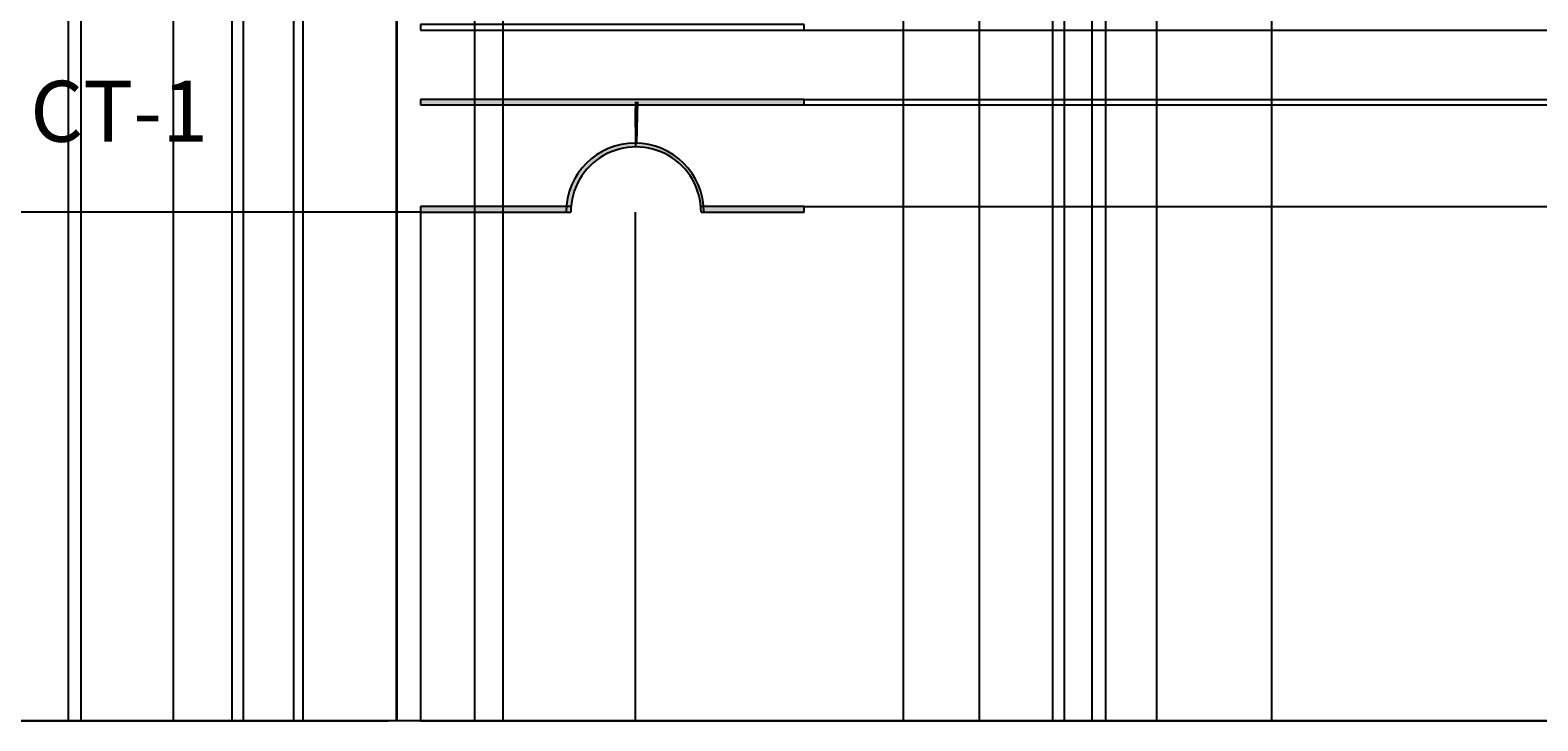
# Model space of a CAD drawing. Units: inches. Extents: x 35362 to 73946, y 43607 to 67532.
# Tile 126 of 134: x 52380 to 57838, y 43607 to 46109. Entities that reach past the tile are written whole.
import ezdxf

# ---------------------------------------------------------------- set-up
doc = ezdxf.new("R2010")
doc.units = ezdxf.units.IN
doc.header["$MEASUREMENT"] = 0
for name, color, linetype, lineweight in [('A-ANNO-DIMS', 2, 'Continuous', 18), ('E-ANNO-TEXT', 5, 'Continuous', 18), ('E-SYMB', 1, 'Continuous', 25), ('E-SYMB-PATT', 1, 'Continuous', 13)]:
    doc.layers.add(name, color=color, linetype=linetype, lineweight=lineweight)
doc.styles.get("Standard").update_dxf_attribs({"font": 'arial.ttf'})
doc.dimstyles.get("Standard").update_dxf_attribs({"dimtxt": 0.18, "dimasz": 0.18, "dimexe": 0.18, "dimexo": 0.0625, "dimgap": 0.09, "dimtad": 0, "dimtih": 1, "dimtoh": 1, "dimdec": 4, "dimzin": 0, "dimdsep": 46, "dimtxsty": 'Standard', "dimcen": 0.09, "dimadec": 0, "dimazin": 0, "dimtfac": 1, "dimtdec": 4, "dimtofl": 0, "dimtmove": 0, "dimatfit": 3, "dimfxl": 1, "dimtolj": 1, "dimtzin": 0, "dimarcsym": 0})

# ---------------------------------------------------------------- blocks, each defined once
blk = doc.blocks.new('CT-CORE')
for p, q in [((0, 1388), (0, 0)), ((20, 1388), (0, 1388)), ((20, 0), (20, 1388)), ((270.7, 1388), (270.7, 0)), ((290.7, 1388), (270.7, 1388)), ((290.7, 0), (290.7, 1388)), ((659, 1388), (659, 1014.6)), ((679, 1388), (659, 1388)), ((679, 1015.4), (679, 1388)), ((659, 544.4), (659, 0)), ((679, 0), (679, 543.5)), ((0, 0), (20, 0)), ((270.7, 0), (290.7, 0)), ((659, 0), (679, 0))]:
    blk.add_line(p, q)
blk.add_arc((679, 779.5), 235.9, 90, 270)
blk = doc.blocks.new('*D5')
at = {"layer": 'A-ANNO-DIMS', "color": 0, "lineweight": -2, "transparency": 16777216}
for p, q in [((37121.9, 46919.3), (37121.9, 43606.7)), ((69871.5, 45449.8), (69871.5, 43606.7)), ((37122.1, 43606.9), (53496.3, 43606.9)), ((69871.3, 43606.9), (53497.2, 43606.9))]:
    blk.add_line(p, q, dxfattribs=at)
at = {"layer": 'A-ANNO-DIMS', "color": 0, "transparency": 16777216}
for points in [[(37122.1, 43606.9), (37122.1, 43606.8), (37121.9, 43606.9)], [(69871.3, 43606.9), (69871.3, 43606.8), (69871.5, 43606.9)]]:
    blk.add_solid(points, dxfattribs=at)
at = {"layer": 'Defpoints', "color": 0, "transparency": 16777216}
for p in [(37121.9, 46919.4), (69871.5, 45449.9), (69871.5, 43606.9)]:
    blk.add_point(p, dxfattribs=at)
at = {"layer": 'A-ANNO-DIMS', "color": 0, "transparency": 16777216, "insert": (53496.7, 43606.9), "char_height": 0.18, "attachment_point": 5}
blk.add_mtext('\\A1;32750', dxfattribs=at)
blk = doc.blocks.new('*D11')
at = {"layer": 'A-ANNO-DIMS', "color": 0, "lineweight": -2, "transparency": 16777216}
for p, q in [((47978.7, 56028.8), (47978.7, 43606.7)), ((53109.8, 56028.8), (53109.8, 43606.7)), ((47978.8, 43606.9), (50543.9, 43606.9)), ((53109.6, 43606.9), (50544.6, 43606.9))]:
    blk.add_line(p, q, dxfattribs=at)
at = {"layer": 'A-ANNO-DIMS', "color": 0, "transparency": 16777216}
for points in [[(47978.8, 43606.9), (47978.8, 43606.8), (47978.7, 43606.9)], [(53109.6, 43606.9), (53109.6, 43606.8), (53109.8, 43606.9)]]:
    blk.add_solid(points, dxfattribs=at)
at = {"layer": 'Defpoints', "color": 0, "transparency": 16777216}
for p in [(47978.7, 56028.8), (53109.8, 56028.8), (53109.8, 43606.9)]:
    blk.add_point(p, dxfattribs=at)
at = {"layer": 'A-ANNO-DIMS', "color": 0, "transparency": 16777216, "insert": (50544.2, 43606.9), "char_height": 0.18, "attachment_point": 5}
blk.add_mtext('\\A1;5131', dxfattribs=at)
blk = doc.blocks.new('*D37')
at = {"layer": 'A-ANNO-DIMS', "color": 0, "lineweight": -2, "transparency": 16777216}
for p, q in [((53793.6, 45449.8), (53793.6, 43606.7)), ((62090.6, 45366.8), (62090.6, 43606.7)), ((53793.8, 43606.9), (57941.6, 43606.9)), ((62090.4, 43606.9), (57942.6, 43606.9))]:
    blk.add_line(p, q, dxfattribs=at)
at = {"layer": 'A-ANNO-DIMS', "color": 0, "transparency": 16777216}
for points in [[(53793.8, 43606.9), (53793.8, 43606.8), (53793.6, 43606.9)], [(62090.4, 43606.9), (62090.4, 43606.8), (62090.6, 43606.9)]]:
    blk.add_solid(points, dxfattribs=at)
at = {"layer": 'Defpoints', "color": 0, "transparency": 16777216}
for p in [(53793.6, 45449.9), (62090.6, 45366.9), (62090.6, 43606.9)]:
    blk.add_point(p, dxfattribs=at)
at = {"layer": 'A-ANNO-DIMS', "color": 0, "transparency": 16777216, "insert": (57942.1, 43606.9), "char_height": 0.18, "attachment_point": 5}
blk.add_mtext('\\A1;8296.9', dxfattribs=at)
blk = doc.blocks.new('*D44')
at = {"layer": 'A-ANNO-DIMS', "color": 0, "lineweight": -2, "transparency": 16777216}
for p, q in [((52517.8, 64828.5), (52517.8, 43606.7)), ((54090.8, 64828.5), (54090.8, 43606.7)), ((52518, 43606.9), (53303.8, 43606.9)), ((54090.6, 43606.9), (53304.7, 43606.9))]:
    blk.add_line(p, q, dxfattribs=at)
at = {"layer": 'A-ANNO-DIMS', "color": 0, "transparency": 16777216}
for points in [[(52518, 43606.9), (52518, 43606.8), (52517.8, 43606.9)], [(54090.6, 43606.9), (54090.6, 43606.8), (54090.8, 43606.9)]]:
    blk.add_solid(points, dxfattribs=at)
at = {"layer": 'Defpoints', "color": 0, "transparency": 16777216}
for p in [(52517.8, 64828.6), (54090.8, 64828.6), (54090.8, 43606.9)]:
    blk.add_point(p, dxfattribs=at)
at = {"layer": 'A-ANNO-DIMS', "color": 0, "transparency": 16777216, "insert": (53304.3, 43606.9), "char_height": 0.18, "attachment_point": 5}
blk.add_mtext('\\A1;1573.0', dxfattribs=at)
blk = doc.blocks.new('*D49')
at = {"layer": 'A-ANNO-DIMS', "color": 0, "lineweight": -2, "transparency": 16777216}
for p, q in [((56457.3, 54249.8), (56457.3, 43606.7)), ((56873.6, 54249.8), (56873.6, 43606.7)), ((56457.5, 43606.9), (56665, 43606.9)), ((56873.4, 43606.9), (56665.8, 43606.9))]:
    blk.add_line(p, q, dxfattribs=at)
at = {"layer": 'A-ANNO-DIMS', "color": 0, "transparency": 16777216}
for points in [[(56457.5, 43606.9), (56457.5, 43606.8), (56457.3, 43606.9)], [(56873.4, 43606.9), (56873.4, 43606.8), (56873.6, 43606.9)]]:
    blk.add_solid(points, dxfattribs=at)
at = {"layer": 'Defpoints', "color": 0, "transparency": 16777216}
for p in [(56457.3, 54249.8), (56873.6, 54249.8), (56873.6, 43606.9)]:
    blk.add_point(p, dxfattribs=at)
at = {"layer": 'A-ANNO-DIMS', "color": 0, "transparency": 16777216, "insert": (56665.4, 43606.9), "char_height": 0.18, "attachment_point": 5}
blk.add_mtext('\\A1;416.3', dxfattribs=at)
blk = doc.blocks.new('*D53')
at = {"layer": 'A-ANNO-DIMS', "color": 0, "lineweight": -2, "transparency": 16777216}
for p, q in [((56873.6, 53351.5), (56873.6, 43606.7)), ((58224.8, 52935.2), (58224.8, 43606.7)), ((56873.8, 43606.9), (57548.7, 43606.9)), ((58224.6, 43606.9), (57549.6, 43606.9))]:
    blk.add_line(p, q, dxfattribs=at)
at = {"layer": 'A-ANNO-DIMS', "color": 0, "transparency": 16777216}
for points in [[(56873.8, 43606.9), (56873.8, 43606.8), (56873.6, 43606.9)], [(58224.6, 43606.9), (58224.6, 43606.8), (58224.8, 43606.9)]]:
    blk.add_solid(points, dxfattribs=at)
at = {"layer": 'Defpoints', "color": 0, "transparency": 16777216}
for p in [(56873.6, 53351.5), (58224.8, 52935.2), (58224.8, 43606.9)]:
    blk.add_point(p, dxfattribs=at)
at = {"layer": 'A-ANNO-DIMS', "color": 0, "transparency": 16777216, "insert": (57549.2, 43606.9), "char_height": 0.18, "attachment_point": 5}
blk.add_mtext('\\A1;1351.2', dxfattribs=at)
blk = doc.blocks.new('*D64')
at = {"layer": 'A-ANNO-DIMS', "color": 0, "lineweight": -2, "transparency": 16777216}
for p, q in [((54578.1, 45848.9), (54575, 45699.4)), ((54578.3, 45848.9), (54578.1, 45848.9)), ((54569.7, 45449.9), (54569.9, 45449.9)), ((54569.8, 45449.8), (54569.8, 45450))]:
    blk.add_line(p, q, dxfattribs=at)
at = {"layer": 'A-ANNO-DIMS', "color": 0, "transparency": 16777216}
blk.add_solid([(54575, 45699.4), (54575, 45699.4), (54575, 45699.3)], dxfattribs=at)
at = {"layer": 'Defpoints', "color": 0, "transparency": 16777216}
for p in [(54575, 45699.3), (54569.8, 45449.9)]:
    blk.add_point(p, dxfattribs=at)
at = {"layer": 'A-ANNO-DIMS', "color": 0, "transparency": 16777216, "insert": (54579, 45848.9), "char_height": 0.18, "attachment_point": 5}
blk.add_mtext('\\A1;5X R249.4', dxfattribs=at)
blk = doc.blocks.new('*D67')
at = {"layer": 'A-ANNO-DIMS', "color": 0, "lineweight": -2, "transparency": 16777216}
for p, q in [((56873.5, 53351.5), (35361.8, 53351.5)), ((35361.9, 53351.3), (35361.9, 49400.9)), ((35361.9, 45450.1), (35361.9, 49400.5)), ((53793.6, 45449.9), (35361.8, 45449.9))]:
    blk.add_line(p, q, dxfattribs=at)
at = {"layer": 'A-ANNO-DIMS', "color": 0, "transparency": 16777216}
for points in [[(35361.9, 53351.3), (35362, 53351.3), (35361.9, 53351.5)], [(35361.9, 45450.1), (35362, 45450.1), (35361.9, 45449.9)]]:
    blk.add_solid(points, dxfattribs=at)
at = {"layer": 'Defpoints', "color": 0, "transparency": 16777216}
for p in [(35361.9, 53351.5), (56873.6, 53351.5), (53793.6, 45449.9)]:
    blk.add_point(p, dxfattribs=at)
at = {"layer": 'A-ANNO-DIMS', "color": 0, "transparency": 16777216, "insert": (35361.9, 49400.7), "char_height": 0.18, "attachment_point": 5}
blk.add_mtext('\\A1;7901.6', dxfattribs=at)
blk = doc.blocks.new('*D74')
at = {"layer": 'A-ANNO-DIMS', "color": 0, "lineweight": -2, "transparency": 16777216}
for p, q in [((55181.7, 46108.9), (73945.8, 46108.9)), ((73945.6, 46108.7), (73945.6, 45983.7)), ((73945.6, 45858.4), (73945.6, 45983.4)), ((55181.7, 45858.2), (73945.8, 45858.2))]:
    blk.add_line(p, q, dxfattribs=at)
at = {"layer": 'A-ANNO-DIMS', "color": 0, "transparency": 16777216}
for points in [[(73945.6, 46108.7), (73945.7, 46108.7), (73945.6, 46108.9)], [(73945.6, 45858.4), (73945.7, 45858.4), (73945.6, 45858.2)]]:
    blk.add_solid(points, dxfattribs=at)
at = {"layer": 'Defpoints', "color": 0, "transparency": 16777216}
for p in [(55181.6, 46108.9), (55181.6, 45858.2), (73945.6, 45858.2)]:
    blk.add_point(p, dxfattribs=at)
at = {"layer": 'A-ANNO-DIMS', "color": 0, "transparency": 16777216, "insert": (73945.6, 45983.5), "char_height": 0.18, "attachment_point": 5}
blk.add_mtext('\\A1;250.67', dxfattribs=at)
blk = doc.blocks.new('*D75')
at = {"layer": 'A-ANNO-DIMS', "color": 0, "lineweight": -2, "transparency": 16777216}
for p, q in [((55181.7, 45838.2), (73945.8, 45838.2)), ((73945.6, 45838), (73945.6, 45654.2)), ((73945.6, 45470.1), (73945.6, 45653.9)), ((55181.7, 45469.9), (73945.8, 45469.9))]:
    blk.add_line(p, q, dxfattribs=at)
at = {"layer": 'A-ANNO-DIMS', "color": 0, "transparency": 16777216}
for points in [[(73945.6, 45838), (73945.7, 45838), (73945.6, 45838.2)], [(73945.6, 45470.1), (73945.7, 45470.1), (73945.6, 45469.9)]]:
    blk.add_solid(points, dxfattribs=at)
at = {"layer": 'Defpoints', "color": 0, "transparency": 16777216}
for p in [(55181.6, 45838.2), (55181.6, 45469.9), (73945.6, 45469.9)]:
    blk.add_point(p, dxfattribs=at)
at = {"layer": 'A-ANNO-DIMS', "color": 0, "transparency": 16777216, "insert": (73945.6, 45654.1), "char_height": 0.18, "attachment_point": 5}
blk.add_mtext('\\A1;368.3', dxfattribs=at)
blk = doc.blocks.new('*D81')
at = {"layer": 'A-ANNO-DIMS', "color": 0, "lineweight": -2, "transparency": 16777216}
for p, q in [((53793.6, 45449.8), (53793.6, 43606.7)), ((54569.8, 45449.8), (54569.8, 43606.7)), ((53793.8, 43606.9), (54181.3, 43606.9)), ((54569.6, 43606.9), (54182.1, 43606.9))]:
    blk.add_line(p, q, dxfattribs=at)
at = {"layer": 'A-ANNO-DIMS', "color": 0, "transparency": 16777216}
for points in [[(53793.8, 43606.9), (53793.8, 43606.8), (53793.6, 43606.9)], [(54569.6, 43606.9), (54569.6, 43606.8), (54569.8, 43606.9)]]:
    blk.add_solid(points, dxfattribs=at)
at = {"layer": 'Defpoints', "color": 0, "transparency": 16777216}
for p in [(53793.6, 45449.9), (54569.8, 45449.9), (54569.8, 43606.9)]:
    blk.add_point(p, dxfattribs=at)
at = {"layer": 'A-ANNO-DIMS', "color": 0, "transparency": 16777216, "insert": (54181.7, 43606.9), "char_height": 0.18, "attachment_point": 5}
blk.add_mtext('\\A1;776.1', dxfattribs=at)
blk = doc.blocks.new('*D83')
at = {"layer": 'A-ANNO-DIMS', "color": 0, "lineweight": -2, "transparency": 16777216}
for p, q in [((55815.3, 49110), (55815.3, 43606.7)), ((55540.3, 48969.9), (55540.3, 43606.7)), ((55540.5, 43606.9), (55677.4, 43606.9)), ((55815.1, 43606.9), (55678.2, 43606.9))]:
    blk.add_line(p, q, dxfattribs=at)
at = {"layer": 'A-ANNO-DIMS', "color": 0, "transparency": 16777216}
for points in [[(55540.5, 43606.9), (55540.5, 43606.8), (55540.3, 43606.9)], [(55815.1, 43606.9), (55815.1, 43606.8), (55815.3, 43606.9)]]:
    blk.add_solid(points, dxfattribs=at)
at = {"layer": 'Defpoints', "color": 0, "transparency": 16777216}
for p in [(55815.3, 49110.1), (55540.3, 48970), (55815.3, 43606.9)]:
    blk.add_point(p, dxfattribs=at)
at = {"layer": 'A-ANNO-DIMS', "color": 0, "transparency": 16777216, "insert": (55677.8, 43606.9), "char_height": 0.18, "attachment_point": 5}
blk.add_mtext('\\A1;275.0', dxfattribs=at)
blk = doc.blocks.new('*D91')
at = {"layer": 'A-ANNO-DIMS', "color": 0, "lineweight": -2, "transparency": 16777216}
for p, q in [((52563.1, 48897.7), (52563.1, 43606.7)), ((53707.8, 48897.7), (53707.8, 43606.7)), ((52563.3, 43606.9), (53135, 43606.9)), ((53707.6, 43606.9), (53135.9, 43606.9))]:
    blk.add_line(p, q, dxfattribs=at)
at = {"layer": 'A-ANNO-DIMS', "color": 0, "transparency": 16777216}
for points in [[(52563.3, 43606.9), (52563.3, 43606.8), (52563.1, 43606.9)], [(53707.6, 43606.9), (53707.6, 43606.8), (53707.8, 43606.9)]]:
    blk.add_solid(points, dxfattribs=at)
at = {"layer": 'Defpoints', "color": 0, "transparency": 16777216}
for p in [(52563.1, 48897.7), (53707.8, 48897.7), (53707.8, 43606.9)]:
    blk.add_point(p, dxfattribs=at)
at = {"layer": 'A-ANNO-DIMS', "color": 0, "transparency": 16777216, "insert": (53135.5, 43606.9), "char_height": 0.18, "attachment_point": 5}
blk.add_mtext('\\A1;1144.6', dxfattribs=at)
blk = doc.blocks.new('*D96')
at = {"layer": 'A-ANNO-DIMS', "color": 0, "lineweight": -2, "transparency": 16777216}
for p, q in [((53366.8, 64997.6), (53366.8, 43606.7)), ((53988.6, 64997.6), (53988.6, 43606.7)), ((53366.9, 43606.9), (53677.3, 43606.9)), ((53988.4, 43606.9), (53678.1, 43606.9))]:
    blk.add_line(p, q, dxfattribs=at)
at = {"layer": 'A-ANNO-DIMS', "color": 0, "transparency": 16777216}
for points in [[(53366.9, 43606.9), (53366.9, 43606.8), (53366.8, 43606.9)], [(53988.4, 43606.9), (53988.4, 43606.8), (53988.6, 43606.9)]]:
    blk.add_solid(points, dxfattribs=at)
at = {"layer": 'Defpoints', "color": 0, "transparency": 16777216}
for p in [(53366.8, 64997.7), (53988.6, 64997.7), (53988.6, 43606.9)]:
    blk.add_point(p, dxfattribs=at)
at = {"layer": 'A-ANNO-DIMS', "color": 0, "transparency": 16777216, "insert": (53677.7, 43606.9), "char_height": 0.18, "attachment_point": 5}
blk.add_mtext('\\A1;621.8', dxfattribs=at)
blk = doc.blocks.new('*D99')
at = {"layer": 'A-ANNO-DIMS', "color": 0, "lineweight": -2, "transparency": 16777216}
for p, q in [((52897.5, 65291.5), (52897.5, 43606.7)), ((52517.8, 64828.5), (52517.8, 43606.7)), ((52518, 43606.9), (52707.2, 43606.9)), ((52897.3, 43606.9), (52708, 43606.9))]:
    blk.add_line(p, q, dxfattribs=at)
at = {"layer": 'A-ANNO-DIMS', "color": 0, "transparency": 16777216}
for points in [[(52518, 43606.9), (52518, 43606.8), (52517.8, 43606.9)], [(52897.3, 43606.9), (52897.3, 43606.8), (52897.5, 43606.9)]]:
    blk.add_solid(points, dxfattribs=at)
at = {"layer": 'Defpoints', "color": 0, "transparency": 16777216}
for p in [(52897.5, 65291.6), (52517.8, 64828.6), (52897.5, 43606.9)]:
    blk.add_point(p, dxfattribs=at)
at = {"layer": 'A-ANNO-DIMS', "color": 0, "transparency": 16777216, "insert": (52707.6, 43606.9), "char_height": 0.18, "attachment_point": 5}
blk.add_mtext('\\A1;379.7', dxfattribs=at)
blk = doc.blocks.new('*D100')
at = {"layer": 'A-ANNO-DIMS', "color": 0, "lineweight": -2, "transparency": 16777216}
for p, q in [((52897.5, 65291.5), (52897.5, 43606.7)), ((53150.7, 64926.1), (53150.7, 43606.7)), ((52897.7, 43606.9), (53023.7, 43606.9)), ((53150.5, 43606.9), (53024.5, 43606.9))]:
    blk.add_line(p, q, dxfattribs=at)
at = {"layer": 'A-ANNO-DIMS', "color": 0, "transparency": 16777216}
for points in [[(52897.7, 43606.9), (52897.7, 43606.8), (52897.5, 43606.9)], [(53150.5, 43606.9), (53150.5, 43606.8), (53150.7, 43606.9)]]:
    blk.add_solid(points, dxfattribs=at)
at = {"layer": 'Defpoints', "color": 0, "transparency": 16777216}
for p in [(52897.5, 65291.6), (53150.7, 64926.1), (53150.7, 43606.9)]:
    blk.add_point(p, dxfattribs=at)
at = {"layer": 'A-ANNO-DIMS', "color": 0, "transparency": 16777216, "insert": (53024.1, 43606.9), "char_height": 0.18, "attachment_point": 5}
blk.add_mtext('\\A1;253.2', dxfattribs=at)
blk = doc.blocks.new('*D102')
at = {"layer": 'A-ANNO-DIMS', "color": 0, "lineweight": -2, "transparency": 16777216}
for p, q in [((56080.5, 63694.7), (56080.5, 43606.7)), ((56272.5, 63696.8), (56272.5, 43606.7)), ((56080.7, 43606.9), (56176, 43606.9)), ((56272.3, 43606.9), (56176.9, 43606.9))]:
    blk.add_line(p, q, dxfattribs=at)
at = {"layer": 'A-ANNO-DIMS', "color": 0, "transparency": 16777216}
for points in [[(56080.7, 43606.9), (56080.7, 43606.8), (56080.5, 43606.9)], [(56272.3, 43606.9), (56272.3, 43606.8), (56272.5, 43606.9)]]:
    blk.add_solid(points, dxfattribs=at)
at = {"layer": 'Defpoints', "color": 0, "transparency": 16777216}
for p in [(56080.5, 63694.8), (56272.5, 63696.9), (56272.5, 43606.9)]:
    blk.add_point(p, dxfattribs=at)
at = {"layer": 'A-ANNO-DIMS', "color": 0, "transparency": 16777216, "insert": (56176.5, 43606.9), "char_height": 0.18, "attachment_point": 5}
blk.add_mtext('\\A1;191.98', dxfattribs=at)
blk = doc.blocks.new('*D104')
at = {"layer": 'A-ANNO-DIMS', "color": 0, "lineweight": -2, "transparency": 16777216}
for p, q in [((56123.2, 63318.1), (56123.2, 43606.7)), ((56223, 63318.1), (56223, 43606.7)), ((56123.4, 43606.9), (56172.7, 43606.9)), ((56222.8, 43606.9), (56173.5, 43606.9))]:
    blk.add_line(p, q, dxfattribs=at)
at = {"layer": 'A-ANNO-DIMS', "color": 0, "transparency": 16777216}
for points in [[(56123.4, 43606.9), (56123.4, 43606.8), (56123.2, 43606.9)], [(56222.8, 43606.9), (56222.8, 43606.8), (56223, 43606.9)]]:
    blk.add_solid(points, dxfattribs=at)
at = {"layer": 'Defpoints', "color": 0, "transparency": 16777216}
for p in [(56123.2, 63318.1), (56223, 63318.1), (56223, 43606.9)]:
    blk.add_point(p, dxfattribs=at)
at = {"layer": 'A-ANNO-DIMS', "color": 0, "transparency": 16777216, "insert": (56173.1, 43606.9), "char_height": 0.18, "attachment_point": 5}
blk.add_mtext('\\A1;99.74', dxfattribs=at)
blk = doc.blocks.new('*D112')
at = {"layer": 'A-ANNO-DIMS', "color": 0, "lineweight": -2, "transparency": 16777216}
for p, q in [((53332.8, 60113.4), (53332.8, 43606.7)), ((53705.4, 60126.2), (53705.4, 43606.7)), ((53332.9, 43606.9), (53518.7, 43606.9)), ((53705.2, 43606.9), (53519.5, 43606.9))]:
    blk.add_line(p, q, dxfattribs=at)
at = {"layer": 'A-ANNO-DIMS', "color": 0, "transparency": 16777216}
for points in [[(53332.9, 43606.9), (53332.9, 43606.8), (53332.8, 43606.9)], [(53705.2, 43606.9), (53705.2, 43606.8), (53705.4, 43606.9)]]:
    blk.add_solid(points, dxfattribs=at)
at = {"layer": 'Defpoints', "color": 0, "transparency": 16777216}
for p in [(53332.8, 60113.5), (53705.4, 60126.3), (53705.4, 43606.9)]:
    blk.add_point(p, dxfattribs=at)
at = {"layer": 'A-ANNO-DIMS', "color": 0, "transparency": 16777216, "insert": (53519.1, 43606.9), "char_height": 0.18, "attachment_point": 5}
blk.add_mtext('\\A1;372.6', dxfattribs=at)
blk = doc.blocks.new('*D115')
at = {"layer": 'A-ANNO-DIMS', "color": 0, "lineweight": -2, "transparency": 16777216}
for p, q in [((54571.7, 45849), (54571, 45699.5)), ((54571.9, 45849), (54571.7, 45849)), ((54569.7, 45449.9), (54569.9, 45449.9)), ((54569.8, 45449.8), (54569.8, 45450))]:
    blk.add_line(p, q, dxfattribs=at)
at = {"layer": 'A-ANNO-DIMS', "color": 0, "transparency": 16777216}
blk.add_solid([(54571, 45699.5), (54571, 45699.5), (54571, 45699.3)], dxfattribs=at)
at = {"layer": 'Defpoints', "color": 0, "transparency": 16777216}
for p in [(54571, 45699.3), (54569.8, 45449.9)]:
    blk.add_point(p, dxfattribs=at)
at = {"layer": 'A-ANNO-DIMS', "color": 0, "transparency": 16777216, "insert": (54572.6, 45849), "char_height": 0.18, "attachment_point": 5}
blk.add_mtext('\\A1;5X R249.4', dxfattribs=at)
blk = doc.blocks.new('*D116')
at = {"layer": 'A-ANNO-DIMS', "color": 0, "lineweight": -2, "transparency": 16777216}
for p, q in [((54569.5, 45827.4), (54569.7, 45827.4)), ((54569.7, 45827.4), (54571, 45686)), ((54573, 45449.9), (54573.2, 45449.9)), ((54573.1, 45449.8), (54573.1, 45450))]:
    blk.add_line(p, q, dxfattribs=at)
at = {"layer": 'A-ANNO-DIMS', "color": 0, "transparency": 16777216}
blk.add_solid([(54571, 45686), (54571, 45686), (54571, 45685.8)], dxfattribs=at)
at = {"layer": 'Defpoints', "color": 0, "transparency": 16777216}
for p in [(54571, 45685.8), (54573.1, 45449.9)]:
    blk.add_point(p, dxfattribs=at)
at = {"layer": 'A-ANNO-DIMS', "color": 0, "transparency": 16777216, "insert": (54568.8, 45827.4), "char_height": 0.18, "attachment_point": 5}
blk.add_mtext('\\A1;5X R235.95', dxfattribs=at)

msp = doc.modelspace()

# ---------------------------------------------------------------- hatches: boundary and pattern name
at = {"layer": 'E-SYMB-PATT'}
h = msp.add_hatch(color=256, dxfattribs=at)
h.dxf.hatch_style = 1
h.paths.add_polyline_path([(55181.634, 45838.209), (55181.634, 45858.209), (53793.638, 45858.209), (53793.638, 45838.209)])
h = msp.add_hatch(color=256, dxfattribs=at)
h.dxf.hatch_style = 1
h.paths.add_polyline_path([(54808.223, 45469.894), (54818.379, 45469.894, 0.39089292), (54569.764, 45699.313, 0.39089292), (54321.149, 45469.894), (54338.022, 45469.894, -0.38956985), (54573.123, 45685.844, -0.38956985)])
h = msp.add_hatch(color=256, dxfattribs=at)
h.dxf.hatch_style = 1
h.paths.add_polyline_path([(54337.173, 45449.894, -0.0212196), (54338.022, 45469.894), (54321.149, 45469.894, 0.0200709), (54320.346, 45449.894)])
h.paths.add_polyline_path([(54320.346, 45449.894, -0.0200709), (54321.149, 45469.894), (53793.638, 45469.894), (53793.638, 45449.894)])
h.paths.add_polyline_path([(55181.634, 45449.894), (55181.634, 45469.894), (54818.379, 45469.894, -0.0200709), (54819.182, 45449.894)])
h.paths.add_polyline_path([(54819.182, 45449.894, 0.0200709), (54818.379, 45469.894), (54808.223, 45469.894, -0.0212196), (54809.072, 45449.894)])

# ---------------------------------------------------------------- linework, layer by layer
at = {"layer": 'E-SYMB'}
msp.add_arc((54569.764, 45449.894), 249.418, 0, 180, dxfattribs=at)

# ---------------------------------------------------------------- block references
at = {"layer": 'E-SYMB', "rotation": 269.9999999999965}
msp.add_blockref('CT-CORE', (53793.638, 46128.877), dxfattribs=at)

# ---------------------------------------------------------------- texts
at = {"layer": 'E-ANNO-TEXT'}
msp.add_text('CT-1', height=220.866, dxfattribs=at).set_placement((52379.821, 45704.439))

# ---------------------------------------------------------------- dimensions: what is measured, and where the dimension line sits
at = {"layer": 'A-ANNO-DIMS'}
for base, p1, p2, override, picture, middle in [((52897.48, 43606.859), (52517.798, 64828.556), (52897.48, 65291.589), {"dimdec": 1, "dimlfac": 1, "dimrnd": 0, "dimzin": 0, "dimdsep": 46, "dimlunit": 2}, '*D99', (52707.639, 43606.859)), ((53150.662, 43606.859), (52897.48, 65291.589), (53150.662, 64926.138), {"dimdec": 1, "dimlfac": 1, "dimrnd": 0, "dimzin": 0, "dimdsep": 46, "dimlunit": 2}, '*D100', (53024.071, 43606.859)), ((53988.6156, 43606.859), (53366.7657, 64997.6827), (53988.6156, 64997.6827), {"dimdec": 1, "dimlfac": 1, "dimrnd": 0, "dimzin": 0, "dimdsep": 46, "dimlunit": 2}, '*D96', (53677.6907, 43606.859)), ((54090.768, 43606.859), (52517.798, 64828.556), (54090.768, 64828.556), {"dimdec": 1, "dimlfac": 1, "dimrnd": 0, "dimzin": 0, "dimdsep": 46, "dimlunit": 2}, '*D44', (53304.283, 43606.859)), ((56272.469, 43606.859), (56080.488, 63694.755), (56272.469, 63696.867), {"dimdec": 2, "dimlfac": 1, "dimrnd": 0, "dimzin": 0, "dimdsep": 46, "dimlunit": 2}, '*D102', (56176.479, 43606.859)), ((56222.953, 43606.859), (56123.213, 63318.132), (56222.953, 63318.132), {"dimdec": 2, "dimlfac": 1, "dimrnd": 0, "dimzin": 0, "dimdsep": 46, "dimlunit": 2}, '*D104', (56173.083, 43606.859)), ((53705.36, 43606.859), (53332.762, 60113.464), (53705.36, 60126.3), {"dimdec": 1, "dimlfac": 1, "dimrnd": 0, "dimzin": 0, "dimdsep": 46, "dimlunit": 2}, '*D112', (53519.061, 43606.859)), ((53109.76, 43606.859), (47978.665, 56028.836), (53109.76, 56028.836), {"dimdec": 0, "dimlfac": 1, "dimrnd": 0, "dimzin": 0, "dimdsep": 46, "dimlunit": 2}, '*D11', (50544.212, 43606.859)), ((56873.602, 43606.859), (56457.29, 54249.826), (56873.602, 54249.826), {"dimdec": 1, "dimlfac": 1, "dimrnd": 0, "dimzin": 0, "dimdsep": 46, "dimlunit": 2}, '*D49', (56665.446, 43606.859)), ((58224.785, 43606.859), (56873.602, 53351.529), (58224.785, 52935.216), {"dimdec": 1, "dimlfac": 1, "dimrnd": 0, "dimzin": 0, "dimdsep": 46, "dimlunit": 2}, '*D53', (57549.194, 43606.859)), ((55815.319, 43606.859), (55540.297, 48969.98), (55815.319, 49110.104), {"dimdec": 1, "dimlfac": 1, "dimrnd": 0, "dimzin": 0, "dimdsep": 46, "dimlunit": 2}, '*D83', (55677.808, 43606.859)), ((53707.781, 43606.859), (52563.135, 48897.738), (53707.781, 48897.738), {"dimdec": 1, "dimlfac": 1, "dimrnd": 0, "dimzin": 0, "dimdsep": 46, "dimlunit": 2}, '*D91', (53135.458, 43606.859)), ((69871.496, 43606.859), (37121.949, 46919.381), (69871.496, 45449.894), {"dimdec": 0, "dimlfac": 1, "dimrnd": 0, "dimzin": 0, "dimdsep": 46, "dimlunit": 2}, '*D5', (53496.723, 43606.859)), ((62090.585, 43606.859), (53793.638, 45449.894), (62090.585, 45366.859), {"dimdec": 1, "dimlfac": 1, "dimrnd": 0, "dimzin": 0, "dimdsep": 46, "dimlunit": 2}, '*D37', (57942.111, 43606.859)), ((54569.764, 43606.859), (53793.638, 45449.894), (54569.764, 45449.894), {"dimdec": 1, "dimlfac": 1, "dimrnd": 0, "dimzin": 0, "dimdsep": 46, "dimlunit": 2}, '*D81', (54181.701, 43606.859))]:
    dim = msp.add_linear_dim(base=base, p1=p1, p2=p2, dimstyle='Standard', override=override, dxfattribs=at)
    dim.commit()
    dim.dimension.update_dxf_attribs({"geometry": picture, "text_midpoint": middle})
for base, p1, p2, override, picture, middle in [((35361.949, 53351.529), (53793.638, 45449.894), (56873.602, 53351.529), {"dimdec": 1, "dimlfac": 1, "dimrnd": 0, "dimzin": 0, "dimdsep": 46, "dimlunit": 2}, '*D67', (35361.949, 49400.712)), ((73945.646, 45858.209), (55181.634, 46108.878), (55181.634, 45858.209), {"dimdec": 2, "dimlfac": 1, "dimrnd": 0, "dimzin": 0, "dimdsep": 46, "dimlunit": 2}, '*D74', (73945.646, 45983.543)), ((73945.646, 45469.894), (55181.634, 45838.209), (55181.634, 45469.894), {"dimdec": 1, "dimlfac": 1, "dimrnd": 0, "dimzin": 0, "dimdsep": 46, "dimlunit": 2}, '*D75', (73945.646, 45654.052))]:
    dim = msp.add_linear_dim(base=base, p1=p1, p2=p2, angle=90, dimstyle='Standard', override=override, dxfattribs=at)
    dim.commit()
    dim.dimension.update_dxf_attribs({"geometry": picture, "text_midpoint": middle})
for center, mpoint, override, picture, middle in [((54569.764, 45449.894), (54571.005, 45699.309), {"dimdec": 1, "dimlfac": 1, "dimrnd": 0, "dimzin": 0, "dimdsep": 46, "dimlunit": 2}, '*D115', (54572.602, 45848.958)), ((54569.764, 45449.894), (54574.984, 45699.258), {"dimdec": 1, "dimlfac": 1, "dimrnd": 0, "dimzin": 0, "dimdsep": 46, "dimlunit": 2}, '*D64', (54578.969, 45848.876)), ((54573.123, 45449.894), (54570.992, 45685.834), {"dimdec": 2, "dimlfac": 1, "dimrnd": 0, "dimzin": 0, "dimdsep": 46, "dimlunit": 2}, '*D116', (54568.789, 45827.398))]:
    dim = msp.add_radius_dim(center=center, mpoint=mpoint, text='5X <>', dimstyle='Standard', override=override, dxfattribs=at)
    dim.commit()
    dim.dimension.update_dxf_attribs({"geometry": picture, "text_midpoint": middle, "dimtype": 164})

doc.saveas('drawing.dxf')
